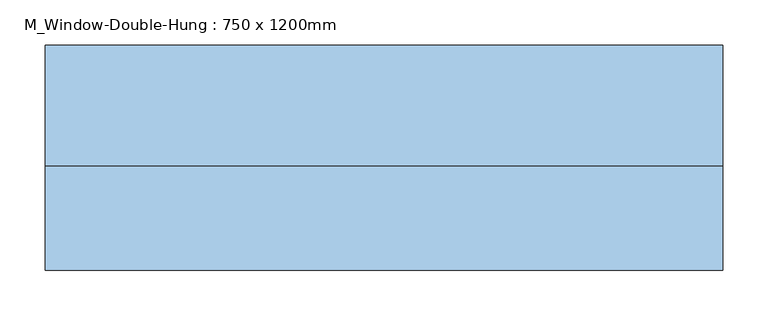
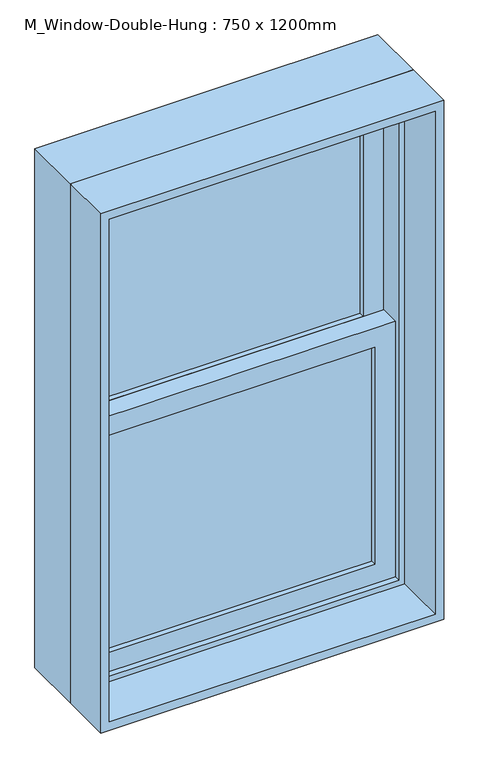
"""IFC4 building model written with IfcOpenShell, lengths in millimetres: window geometry, M_Window-Double-Hung : 750 x 1200mm."""

from ifc_helpers import new_model, si_unit, frame, origin, place, context, project, spatial, polyline, outline, extrude, source, transform, mapped, element, save


def m_window_double_hung_750_x_1200mm_abb80fbd(model_context):
    return source(origin(), model_context, "Body", "SweptSolid", [
        extrude(outline(polyline([(298.8, 45.15), (298.8, 38.8), (-298.8, 38.8), (-298.8, 45.15), (298.8, 45.15)])), frame((0.0, 0.0, 990.6), z_axis=(0.0, 0.0, 1.0), x_axis=(1.0, 0.0, 0.0)), (0.0, 0.0, 1.0), 501.575),
        extrude(outline(polyline([(-298.8, 32.45), (298.8, 32.45), (298.8, 26.1), (-298.8, 26.1), (-298.8, 32.45)])), frame((0.0, 0.0, 990.6), z_axis=(0.0, 0.0, 1.0), x_axis=(1.0, 0.0, 0.0)), (0.0, 0.0, 1.0), 501.575),
        extrude(outline(polyline([(298.8, 89.6), (298.8, 83.25), (-298.8, 83.25), (-298.8, 89.6), (298.8, 89.6)])), frame((0.0, 0.0, 1536.625), z_axis=(0.0, 0.0, 1.0), x_axis=(1.0, 0.0, 0.0)), (0.0, 0.0, 1.0), 501.575),
        extrude(outline(polyline([(-298.8, 76.9), (298.8, 76.9), (298.8, 70.55), (-298.8, 70.55), (-298.8, 76.9)])), frame((0.0, 0.0, 1536.625), z_axis=(0.0, 0.0, 1.0), x_axis=(1.0, 0.0, 0.0)), (0.0, 0.0, 1.0), 501.575),
        extrude(outline(polyline([(1536.625, -343.25), (946.15, -343.25), (946.15, 343.25), (1536.625, 343.25), (1536.625, -343.25)]), holes=[polyline([(1492.175, 298.8), (990.6, 298.8), (990.6, -298.8), (1492.175, -298.8), (1492.175, 298.8)])]), frame((0.0, 13.4, 0.0), z_axis=(0.0, 1.0, 0.0), x_axis=(0.0, 0.0, 1.0)), (0.0, 0.0, 1.0), 44.45),
        extrude(outline(polyline([(2082.65, -343.25), (1492.175, -343.25), (1492.175, 343.25), (2082.65, 343.25), (2082.65, -343.25)]), holes=[polyline([(2038.2, 298.8), (1536.625, 298.8), (1536.625, -298.8), (2038.2, -298.8), (2038.2, 298.8)])]), frame((0.0, 57.85, 0.0), z_axis=(0.0, 1.0, 0.0), x_axis=(0.0, 0.0, 1.0)), (0.0, 0.0, 1.0), 44.45),
        extrude(outline(polyline([(2114.4, -375.0), (914.4, -375.0), (914.4, 375.0), (2114.4, 375.0), (2114.4, -375.0)]), holes=[polyline([(2082.65, 343.25), (946.15, 343.25), (946.15, -343.25), (2082.65, -343.25), (2082.65, 343.25)])]), frame((0.0, 0.7, 0.0), z_axis=(0.0, 1.0, 0.0), x_axis=(0.0, 0.0, 1.0)), (0.0, 0.0, 1.0), 133.35),
        extrude(outline(polyline([(2114.4, 375.0), (2114.4, -375.0), (914.4, -375.0), (914.4, 375.0), (2114.4, 375.0)]), holes=[polyline([(2095.35, 355.95), (933.45, 355.95), (933.45, -355.95), (2095.35, -355.95), (2095.35, 355.95)])]), frame((0.0, -115.0, 0.0), z_axis=(0.0, 1.0, 0.0), x_axis=(0.0, 0.0, 1.0)), (0.0, 0.0, 1.0), 115.7),
    ])


if __name__ == "__main__":
    model = new_model("IFC4")
    model_context = context("Model", 3, world=origin())
    ifc_project = project(units=[si_unit("LENGTHUNIT", "METRE", prefix="MILLI")], contexts=[model_context])
    site = spatial("IfcSite", under=ifc_project)
    building = spatial("IfcBuilding", under=site)
    placement = place(None, origin())
    m_window_double_hung_750_x_1200mm_shape = m_window_double_hung_750_x_1200mm_abb80fbd(model_context)
    element("IfcWindow", 1, ObjectType="M_Window-Double-Hung : 750 x 1200mm", at=placement, inside=building, context=model_context, shape_type="MappedRepresentation", body=[
        mapped(m_window_double_hung_750_x_1200mm_shape, transform((0.0, 0.0, 0.0), x_axis=(1.0, 0.0, 0.0), y_axis=(0.0, 1.0, 0.0), z_axis=(0.0, 0.0, 1.0))),
    ])
    save(model, "model.ifc")

# Revit data of these elements
# Type "M_Window-Double-Hung : 750 x 1200mm"
#   Type Mark = "W2"
#   Fire Rating = "0.5h"
#   Construction Type Id = "DG-DR"
#   Assembly Code = "B2020100"
#   Analytic Construction = "Double glazing - domestic"
#   Wall Thickness [instance default] = 0.15 m
#   Window Inset [instance default] = 0 m
#   Visual Light Transmittance = 0.81
#   Thermal Resistance (R) = 0.319569 (m²·K)/W
#   Solar Heat Gain Coefficient = 0.76
#   Muntin Width = 0.5976 m
#   Muntin Height = 0.501575 m
#   Interior Wall Closure [instance default] = 0.0357 m
#   Rough Width = 0.765 m
#   Rough Height = 1.215 m
#   Frame Extension [instance default] = 0.03175 m
#   Exterior Wall Closure [instance default] = 0.0127 m
#   Extension Jamb [instance default] = 0.0357 m
#   Heat Transfer Coefficient (U) = 3.12929 W/(m²·K)
#   Height = 1.2 m
#   Width = 0.75 m
#   Define Thermal Properties by = 1
#   Top Muntin Visibility = yes
#   Indicator Visibility [instance default] = yes
#   Extension Jamb Visibility [instance default] = yes
#   Interior Trim Visibility [instance default] = yes
#   Exterior Trim Visibility [instance default] = yes
#   Define Thermal Properties by = 1
#   Bottom Muntin Visibility = yes
#   Muntin Pattern = M_Muntin Pattern_2x2 : M_Muntin Pattern_2x2
#   Interior Trim Material = Wood - Stained
#   Interior Trim = M_Trim-Window-Interior-Flat : Picture Frame
#   Exterior Trim Material = Clad - White
#   Exterior Trim = M_Trim-Window-Exterior-Flat : with Sill
#   Glass Panel Material = Glass
#   Exterior Frame Material = Clad - White
#   Interior Frame Material = Wood - Stained
#   Wall Closure = (empty or 0)
# Element 1 (IfcWindow, "M_Window-Double-Hung : 750 x 1200mm")
#   Wall Thickness = 0.23 m
#   Extension Jamb = 0.1157 m
#   Materials on its faces: "Wood - Stained", "Glass", "Clad - White"
# Materials
#   "Wood - Stained": class "Wood", colour RGB 224 178 126, transparency 0, Cost = 0
#   "Clad - White": class "Wood", colour RGB 242 242 238, transparency 0, Cost = 0
#   "Glass": class "Glass", colour RGB 0 128 192, transparency 0.9, Description = "Soda Lime Glass", Cost = 0
